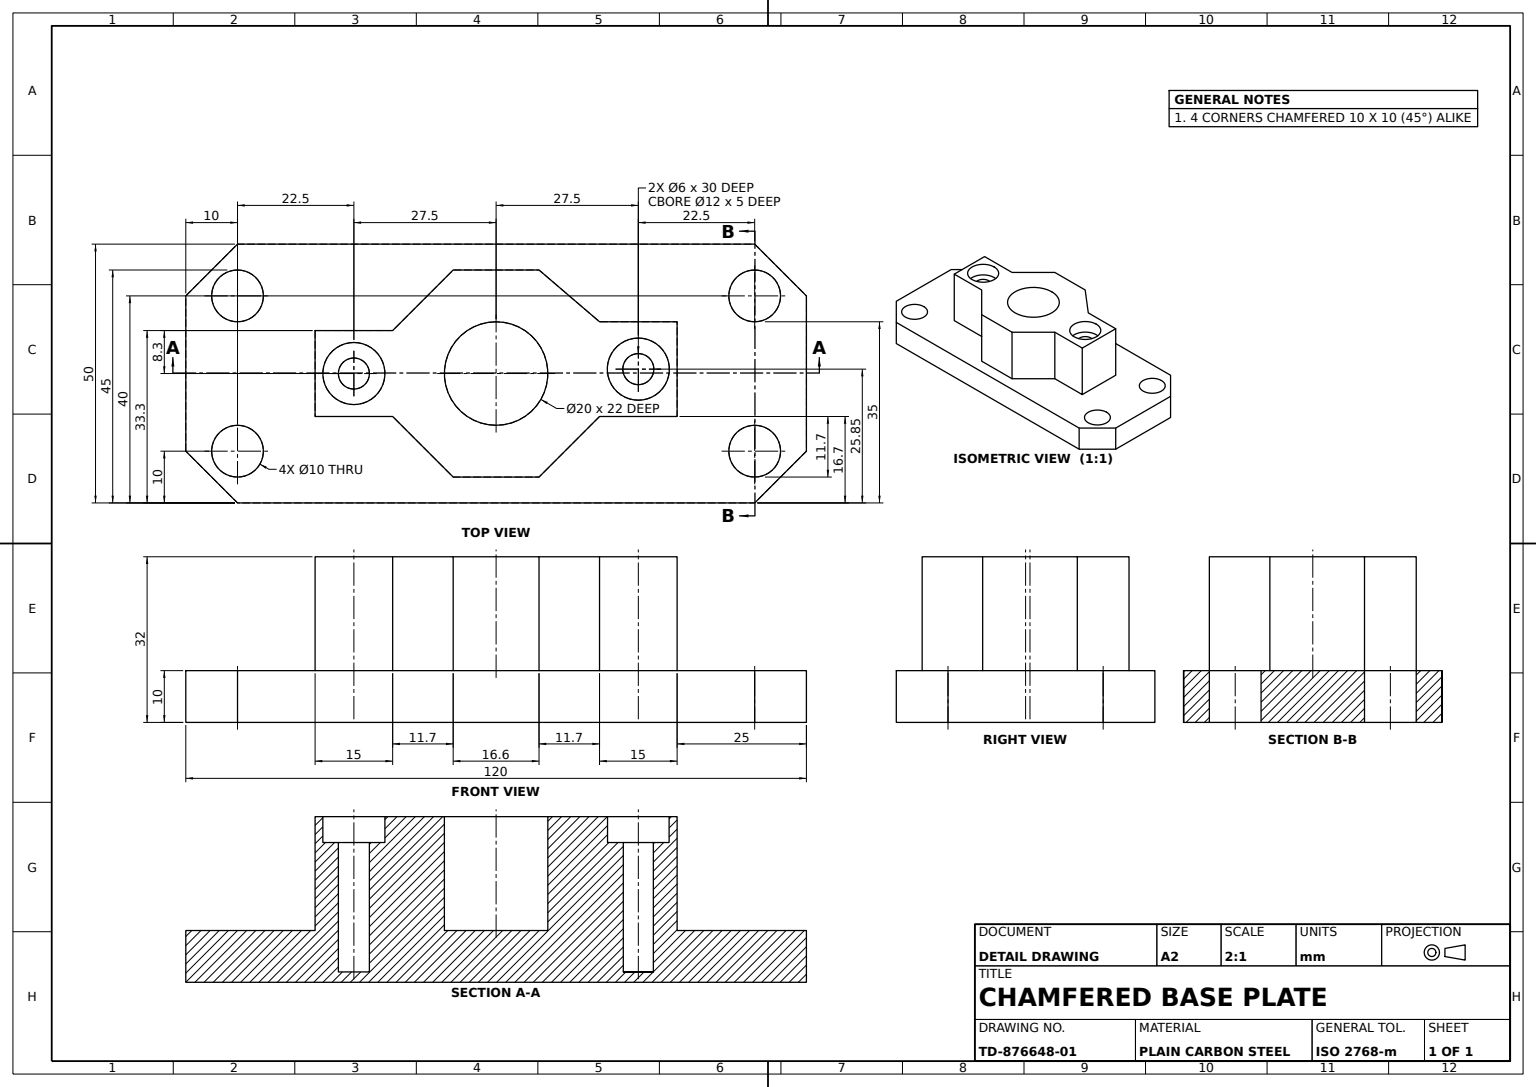
SolidWorks part; units mm, degrees
material "Plain Carbon Steel"
ref_plane "Front Plane" through (0, 0, 0) normal (0, 0, 1) x (1, 0, 0)
ref_plane "Top Plane" through (0, 0, 0) normal (0, 1, 0) x (1, 0, 0)
ref_plane "Right Plane" through (0, 0, 0) normal (1, 0, 0) x (0, 0, -1)
sketch "Base Plate Sketch" plane through (0, 0, 0) normal (0, 0, 1) x (1, 0, 0)
  line L0 (0, 0) -> (120, 0)
  line L1 (120, 0) -> (120, 10)
  line L2 (120, 10) -> (0, 10)
  line L3 (0, 10) -> (0, 0)
  dimension "D1" = 120
  dimension "D2" = 10
extrude "Base Plate" add sketch "Base Plate Sketch" along normal blind 50
sketch "Mounting Holes Sketch" plane through (0, 10, 0) normal (0, 1, 0) x (1, 0, 0)
  line L0 (120, 0) -> (0, 0) construction
  line L1 (0, -50) -> (0, 0) construction
  line L2 (120, -50) -> (120, 0) construction
  line L3 (120, -50) -> (0, -50) construction
  circle A0 centre (10, -10) radius 5
  circle A1 centre (10, -40) radius 5
  circle A2 centre (110, -10) radius 5
  circle A3 centre (110, -40) radius 5
  dimension "D1" = 10
  dimension "D2" = 10
  dimension "D3" = 10
  dimension "D4" = 10
  dimension "D5" = 10
  dimension "D6" = 10
  dimension "D7" = 10
  dimension "D8" = 10
  dimension "D9" = 10
  dimension "D10" = 10
  dimension "D11" = 10
  dimension "D12" = 10
extrude "Mounting Holes 4xØ10" cut sketch "Mounting Holes Sketch" against normal through all
sketch "Center Support Sketch" plane through (0, 10, 0) normal (0, 1, 0) x (1, 0, 0)
  line L2 (10, -5) -> (10, -15) construction
  line L3 (15, -10) -> (5, -10) construction
  line L4 (25, -16.7) -> (40, -16.7)
  line L5 (25, -33.3) -> (40, -33.3)
  line L6 (51.7, -5) -> (68.3, -5)
  line L7 (51.7, -45) -> (68.3, -45)
  line L8 (95, -15) -> (95, -33.3)
  line L11 (25, -16.7) -> (25, -33.3)
  line L14 (51.7, -45) -> (40, -33.3)
  line L15 (40, -16.7) -> (51.7, -5)
  line L17 (95, -15) -> (80, -15)
  line L18 (80, -15) -> (68.3, -5)
  line L20 (95, -33.3) -> (80, -33.3)
  line L21 (80, -33.3) -> (68.3, -45)
  circle A0 centre (10, -10) radius 5 construction
  point P10 (10, -10)
  dimension "D1" = 15
  dimension "D2" = 15
  dimension "D3" = 15
  dimension "D4" = 11.7
  dimension "D5" = 11.7
  dimension "D6" = 16.6
  dimension "D7" = 16.6
  dimension "D8" = 11.7
  dimension "D9" = 11.7
  dimension "D10" = 15
  dimension "D11" = 16.7
  dimension "D12" = 33.3
  dimension "D13" = 5
  dimension "D14" = 15
  dimension "D15" = 45
  dimension "D16" = 33.3
extrude "Center Support" add sketch "Center Support Sketch" along normal blind 22
sketch "Center Bore Sketch" plane through (0, 32, 0) normal (0, 1, 0) x (1, 0, 0)
  line L0 (25, -16.7) -> (25, -33.3) construction
  circle A0 centre (60, -25) radius 10
  dimension "D1" = 20
  dimension "D2" = 35
  dimension "D3" = 8.3
extrude "Center Bore Ø20" cut sketch "Center Bore Sketch" against normal blind 22
sketch "Support Holes Sketch" plane through (0, 32, 0) normal (0, 1, 0) x (1, 0, 0)
  line L0 (25, -16.7) -> (25, -33.3) construction
  circle A0 centre (32.5, -25) radius 3
  circle A1 centre (87.5, -24.15) radius 3
  dimension "D1" = 6
  dimension "D2" = 6
  dimension "D3" = 7.5
  dimension "D4" = 62.5
  dimension "D5" = 8.3
  dimension "D6" = 9.15
extrude "Support Holes 2xØ6" cut sketch "Support Holes Sketch" against normal blind 30
sketch "Counterbore Sketch" plane through (0, 32, 0) normal (0, 1, 0) x (1, 0, 0)
  circle A0 centre (32.5, -25) radius 6
  circle A1 centre (87.5, -24.15) radius 6
  dimension "D1" = 12
  dimension "D2" = 12
extrude "Counterbores 2xØ12x5" cut sketch "Counterbore Sketch" against normal blind 5
chamfer "Corner Chamfers 10mm" distance 10 angle 45 4 edges at (0, 5, 50) (0, 5, 0) (120, 5, 0) (120, 5, 50)
